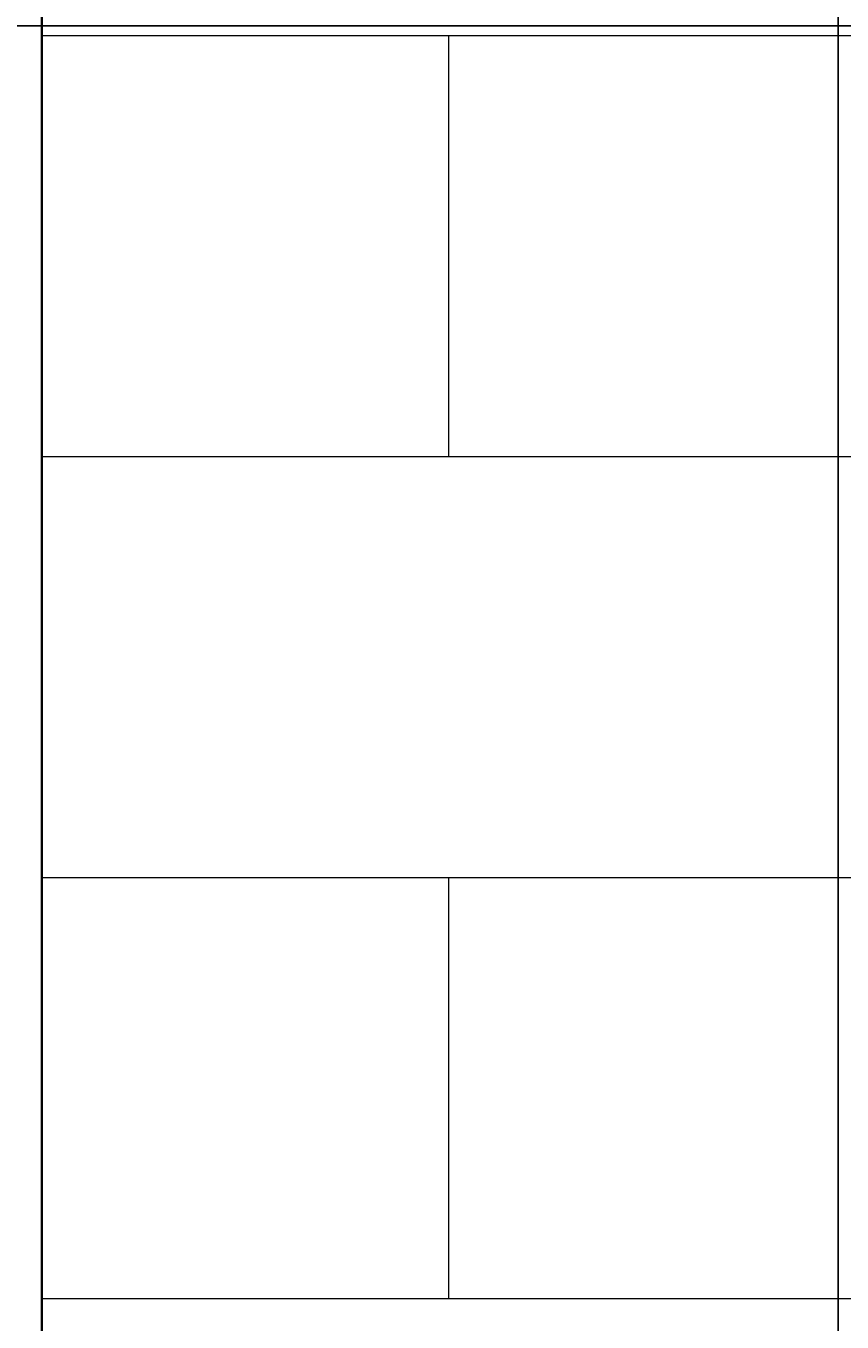
# Model space of a CAD drawing. Units: inches. Extents: x -26 to 776, y -22 to 650.
# Tile 16 of 62: x 288 to 358, y 34 to 145. Entities that reach past the tile are written whole.
import ezdxf

# ---------------------------------------------------------------- set-up
doc = ezdxf.new("R2010")
doc.units = ezdxf.units.IN
doc.header["$MEASUREMENT"] = 0
for name, color, linetype, lineweight in [('A-ANNO-DIMS', 2, 'Continuous', 18), ('A-WALL', 7, 'Continuous', 35), ('A-WALL-PATT', 8, 'Continuous', 13)]:
    doc.layers.add(name, color=color, linetype=linetype, lineweight=lineweight)
doc.styles.get("Standard").update_dxf_attribs({"font": 'arial.ttf'})
doc.dimstyles.get("Standard").update_dxf_attribs({"dimtxt": 0.5625, "dimasz": 0.18, "dimexe": 0.18, "dimexo": 0.0625, "dimgap": 0.09, "dimtad": 0, "dimtih": 1, "dimtoh": 1, "dimdec": 4, "dimzin": 0, "dimdsep": 46, "dimlunit": 4, "dimtxsty": 'Standard', "dimcen": 0.09, "dimadec": 0, "dimazin": 0, "dimtfac": 1, "dimtdec": 4, "dimtofl": 0, "dimtmove": 0, "dimatfit": 3, "dimfxl": 1, "dimtolj": 1, "dimtzin": 0, "dimarcsym": 0})

# ---------------------------------------------------------------- blocks, each defined once
blk = doc.blocks.new('*D13')
at = {"layer": 'A-ANNO-DIMS', "color": 0, "lineweight": -2, "transparency": 16777216}
for p, q in [((738.75, 50.79), (738.75, -21.31)), ((11.11, 15.42), (11.11, -21.31)), ((11.29, -21.13), (373.89, -21.13)), ((738.57, -21.13), (375.97, -21.13))]:
    blk.add_line(p, q, dxfattribs=at)
at = {"layer": 'A-ANNO-DIMS', "color": 0, "transparency": 16777216}
for points in [[(11.29, -21.1), (11.29, -21.16), (11.11, -21.13)], [(738.57, -21.1), (738.57, -21.16), (738.75, -21.13)]]:
    blk.add_solid(points, dxfattribs=at)
at = {"layer": 'Defpoints', "color": 0, "transparency": 16777216}
for p in [(738.75, 50.85), (11.11, 15.48), (738.75, -21.13)]:
    blk.add_point(p, dxfattribs=at)
at = {"layer": 'A-ANNO-DIMS', "color": 0, "transparency": 16777216, "insert": (374.93, -21.13), "char_height": 0.562, "attachment_point": 5}
blk.add_mtext('\\A1;727.6', dxfattribs=at)
blk = doc.blocks.new('*D30')
at = {"layer": 'A-ANNO-DIMS', "color": 0, "lineweight": -2, "transparency": 16777216}
for p, q in [((280.68, 144.84), (775.34, 144.84)), ((775.16, 144.66), (775.16, 86.01)), ((775.16, 26.6), (775.16, 85.25)), ((280.68, 26.42), (775.34, 26.42))]:
    blk.add_line(p, q, dxfattribs=at)
at = {"layer": 'A-ANNO-DIMS', "color": 0, "transparency": 16777216}
for points in [[(775.13, 144.66), (775.19, 144.66), (775.16, 144.84)], [(775.13, 26.6), (775.19, 26.6), (775.16, 26.42)]]:
    blk.add_solid(points, dxfattribs=at)
at = {"layer": 'Defpoints', "color": 0, "transparency": 16777216}
for p in [(280.62, 144.84), (775.16, 144.84), (280.62, 26.42)]:
    blk.add_point(p, dxfattribs=at)
at = {"layer": 'A-ANNO-DIMS', "color": 0, "transparency": 16777216, "insert": (775.16, 85.63), "char_height": 0.562, "attachment_point": 5}
blk.add_mtext('\\A1;118.41', dxfattribs=at)
blk = doc.blocks.new('*D34')
at = {"layer": 'A-ANNO-DIMS', "color": 0, "lineweight": -2, "transparency": 16777216}
for p, q in [((228.57, 528.3), (228.57, -21.31)), ((357.3, 528.36), (357.3, -21.31)), ((228.75, -21.13), (291.71, -21.13)), ((357.12, -21.13), (294.17, -21.13))]:
    blk.add_line(p, q, dxfattribs=at)
at = {"layer": 'A-ANNO-DIMS', "color": 0, "transparency": 16777216}
for points in [[(228.75, -21.1), (228.75, -21.16), (228.57, -21.13)], [(357.12, -21.1), (357.12, -21.16), (357.3, -21.13)]]:
    blk.add_solid(points, dxfattribs=at)
at = {"layer": 'Defpoints', "color": 0, "transparency": 16777216}
for p in [(228.57, 528.36), (357.3, 528.42), (357.3, -21.13)]:
    blk.add_point(p, dxfattribs=at)
at = {"layer": 'A-ANNO-DIMS', "color": 0, "transparency": 16777216, "insert": (292.94, -21.13), "char_height": 0.562, "attachment_point": 5}
blk.add_mtext('\\A1;128.73', dxfattribs=at)
blk = doc.blocks.new('*D39')
at = {"layer": 'A-ANNO-DIMS', "color": 0, "lineweight": -2, "transparency": 16777216}
for p, q in [((289.24, 15.54), (289.24, 649.86)), ((289.42, 649.68), (356.48, 649.68)), ((425.56, 649.68), (358.51, 649.68)), ((425.74, 15.54), (425.74, 649.86))]:
    blk.add_line(p, q, dxfattribs=at)
at = {"layer": 'A-ANNO-DIMS', "color": 0, "transparency": 16777216}
for points in [[(289.42, 649.71), (289.42, 649.65), (289.24, 649.68)], [(425.56, 649.71), (425.56, 649.65), (425.74, 649.68)]]:
    blk.add_solid(points, dxfattribs=at)
at = {"layer": 'Defpoints', "color": 0, "transparency": 16777216}
for p in [(425.74, 649.68), (289.24, 15.48), (425.74, 15.48)]:
    blk.add_point(p, dxfattribs=at)
at = {"layer": 'A-ANNO-DIMS', "color": 0, "transparency": 16777216, "insert": (357.49, 649.68), "char_height": 0.562, "attachment_point": 5}
blk.add_mtext('\\A1;136.5', dxfattribs=at)

msp = doc.modelspace()

# ---------------------------------------------------------------- hatches: boundary and pattern name
at = {"layer": 'A-WALL-PATT'}
h = msp.add_hatch(dxfattribs=at)
h.set_pattern_fill('AR-B816', color=256, scale=4.5)
h.paths.add_polyline_path([(425.7434, 448.2114), (289.2424, 496.9554), (289.2424, 458.1203), (289.2424, 291.1798), (289.2424, 20.7937), (425.7434, 20.7937), (425.7434, 283.2492)])

# ---------------------------------------------------------------- linework, layer by layer
at = {"layer": 'A-WALL'}
for p, q in [((289.2424, 291.1798), (289.2424, 15.4824)), ((289.2424, 15.4824), (289.2424, 159.4824))]:
    msp.add_line(p, q, dxfattribs=at)

# ---------------------------------------------------------------- dimensions: what is measured, and where the dimension line sits
at = {"layer": 'A-ANNO-DIMS'}
for base, p1, p2, override, picture, middle in [((425.7434, 649.6763), (289.2424, 15.4824), (425.7434, 15.4824), {"dimdec": 1, "dimlfac": 1, "dimrnd": 0, "dimzin": 0, "dimdsep": 46, "dimlunit": 2}, '*D39', (357.4929, 649.6763)), ((357.3034, -21.1349), (228.5733, 528.3585), (357.3034, 528.4233), {"dimdec": 2, "dimlfac": 1, "dimrnd": 0, "dimzin": 0, "dimdsep": 46, "dimlunit": 2}, '*D34', (292.9384, -21.1349)), ((738.7503, -21.1349), (11.1074, 15.4824), (738.7503, 50.8482), {"dimdec": 1, "dimlfac": 1, "dimrnd": 0, "dimzin": 0, "dimdsep": 46, "dimlunit": 2}, '*D13', (374.9289, -21.1349))]:
    dim = msp.add_linear_dim(base=base, p1=p1, p2=p2, dimstyle='Standard', override=override, dxfattribs=at)
    dim.commit()
    dim.dimension.update_dxf_attribs({"geometry": picture, "text_midpoint": middle})
dim = msp.add_linear_dim(base=(775.1553, 144.8359), p1=(280.6173, 26.4239), p2=(280.6173, 144.8359), angle=90, dimstyle='Standard', override={"dimdec": 2, "dimlfac": 1, "dimrnd": 0, "dimzin": 0, "dimdsep": 46, "dimlunit": 2}, dxfattribs=at)
dim.commit()
dim.dimension.update_dxf_attribs({"geometry": '*D30', "text_midpoint": (775.1553, 85.6299)})

doc.saveas('drawing.dxf')
